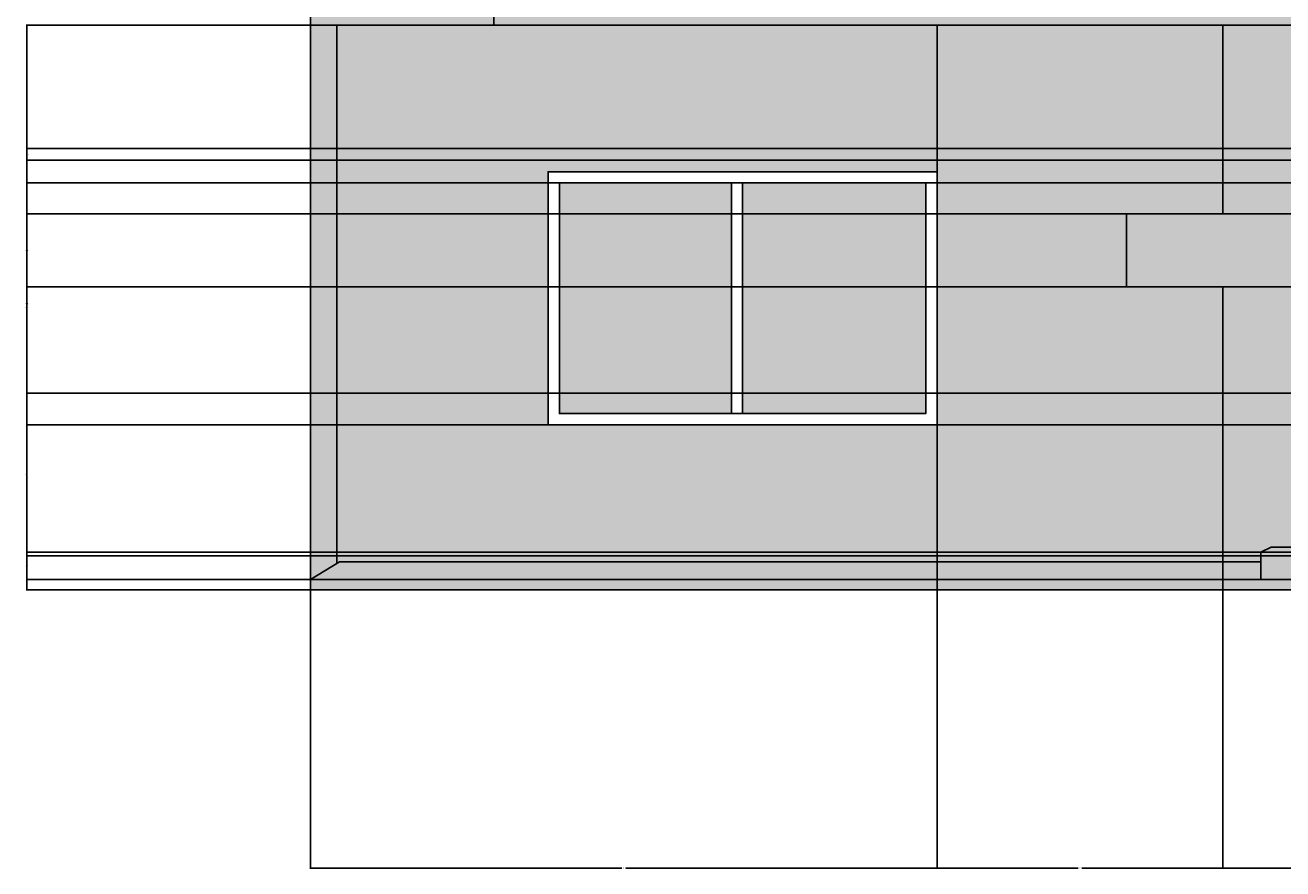
# Model space of a CAD drawing. Units: feet. Extents: x 2193 to 3502, y 890 to 1601.
# Tile 1 of 17: x 2193 to 2466, y 890 to 1073. Entities that reach past the tile are written whole.
import ezdxf

# ---------------------------------------------------------------- set-up
doc = ezdxf.new("R2010")
doc.units = ezdxf.units.FT
for name, color, linetype, lineweight in [('A-ANNO-DIMS', 2, 'Continuous', 18), ('A-ELEV', 7, 'Continuous', 25), ('A-ELEV-PATT', 8, 'Continuous', 13)]:
    doc.layers.add(name, color=color, linetype=linetype, lineweight=lineweight)
doc.styles.get("Standard").update_dxf_attribs({"font": 'arial.ttf'})
doc.dimstyles.get("Standard").update_dxf_attribs({"dimtxt": 0.18, "dimasz": 0.18, "dimexe": 0.18, "dimexo": 0.0625, "dimgap": 0.09, "dimtad": 0, "dimtih": 1, "dimtoh": 1, "dimdec": 0, "dimzin": 0, "dimdsep": 46, "dimlunit": 3, "dimtxsty": 'Standard', "dimcen": 0.09, "dimadec": 0, "dimazin": 0, "dimtfac": 1, "dimtdec": 0, "dimtofl": 0, "dimtmove": 0, "dimatfit": 3, "dimfxl": 1, "dimtolj": 1, "dimtzin": 0, "dimarcsym": 0})

# ---------------------------------------------------------------- blocks, each defined once
blk = doc.blocks.new('*D19')
at = {"layer": 'A-ANNO-DIMS', "color": 0, "lineweight": -2, "transparency": 16777216}
for p, q in [((2934.31, 1073.03), (2193.56, 1073.03)), ((2193.74, 1072.85), (2193.74, 1012.11)), ((2193.74, 951), (2193.74, 1011.75)), ((2934.31, 950.82), (2193.56, 950.82))]:
    blk.add_line(p, q, dxfattribs=at)
at = {"layer": 'A-ANNO-DIMS', "color": 0, "transparency": 16777216}
for points in [[(2193.71, 1072.85), (2193.77, 1072.85), (2193.74, 1073.03)], [(2193.71, 951), (2193.77, 951), (2193.74, 950.82)]]:
    blk.add_solid(points, dxfattribs=at)
at = {"layer": 'Defpoints', "color": 0, "transparency": 16777216}
for p in [(2193.74, 1073.03), (2934.37, 1073.03), (2934.37, 950.82)]:
    blk.add_point(p, dxfattribs=at)
at = {"layer": 'A-ANNO-DIMS', "color": 0, "transparency": 16777216, "insert": (2193.74, 1011.93), "char_height": 0.18, "attachment_point": 5}
blk.add_mtext('\\A1;122.2', dxfattribs=at)
blk = doc.blocks.new('*D23')
at = {"layer": 'A-ANNO-DIMS', "color": 0, "lineweight": -2, "transparency": 16777216}
for p, q in [((2988.24, 1038.87), (2193.56, 1038.87)), ((2193.74, 1038.69), (2193.74, 1012.87)), ((2193.74, 986.69), (2193.74, 1012.51)), ((2985.8, 986.51), (2193.56, 986.51))]:
    blk.add_line(p, q, dxfattribs=at)
at = {"layer": 'A-ANNO-DIMS', "color": 0, "transparency": 16777216}
for points in [[(2193.71, 1038.69), (2193.77, 1038.69), (2193.74, 1038.87)], [(2193.71, 986.69), (2193.77, 986.69), (2193.74, 986.51)]]:
    blk.add_solid(points, dxfattribs=at)
at = {"layer": 'Defpoints', "color": 0, "transparency": 16777216}
for p in [(2193.74, 1038.87), (2988.31, 1038.87), (2985.86, 986.51)]:
    blk.add_point(p, dxfattribs=at)
at = {"layer": 'A-ANNO-DIMS', "color": 0, "transparency": 16777216, "insert": (2193.74, 1012.69), "char_height": 0.18, "attachment_point": 5}
blk.add_mtext('\\A1;52.35', dxfattribs=at)
blk = doc.blocks.new('*D26')
at = {"layer": 'A-ANNO-DIMS', "color": 0, "lineweight": -2, "transparency": 16777216}
for p, q in [((2255.16, 950.89), (2255.16, 1601.47)), ((2255.34, 1601.29), (2507.42, 1601.29)), ((2760.29, 1601.29), (2508.21, 1601.29)), ((2760.47, 1541.11), (2760.47, 1601.47))]:
    blk.add_line(p, q, dxfattribs=at)
at = {"layer": 'A-ANNO-DIMS', "color": 0, "transparency": 16777216}
for points in [[(2255.34, 1601.32), (2255.34, 1601.26), (2255.16, 1601.29)], [(2760.29, 1601.32), (2760.29, 1601.26), (2760.47, 1601.29)]]:
    blk.add_solid(points, dxfattribs=at)
at = {"layer": 'Defpoints', "color": 0, "transparency": 16777216}
for p in [(2760.47, 1601.29), (2760.47, 1541.04), (2255.16, 950.82)]:
    blk.add_point(p, dxfattribs=at)
at = {"layer": 'A-ANNO-DIMS', "color": 0, "transparency": 16777216, "insert": (2507.82, 1601.29), "char_height": 0.18, "attachment_point": 5}
blk.add_mtext('\\A1;505.3', dxfattribs=at)
blk = doc.blocks.new('*D27')
at = {"layer": 'A-ANNO-DIMS', "color": 0, "lineweight": -2, "transparency": 16777216}
for p, q in [((2390.89, 956.87), (2390.89, 890.39)), ((2255.16, 950.76), (2255.16, 890.39)), ((2255.34, 890.57), (2322.57, 890.57)), ((2390.71, 890.57), (2323.48, 890.57))]:
    blk.add_line(p, q, dxfattribs=at)
at = {"layer": 'A-ANNO-DIMS', "color": 0, "transparency": 16777216}
for points in [[(2255.34, 890.6), (2255.34, 890.54), (2255.16, 890.57)], [(2390.71, 890.6), (2390.71, 890.54), (2390.89, 890.57)]]:
    blk.add_solid(points, dxfattribs=at)
at = {"layer": 'Defpoints', "color": 0, "transparency": 16777216}
for p in [(2390.89, 956.94), (2255.16, 950.82), (2390.89, 890.57)]:
    blk.add_point(p, dxfattribs=at)
at = {"layer": 'A-ANNO-DIMS', "color": 0, "transparency": 16777216, "insert": (2323.03, 890.57), "char_height": 0.18, "attachment_point": 5}
blk.add_mtext('\\A1;135.74', dxfattribs=at)
blk = doc.blocks.new('*D28')
at = {"layer": 'A-ANNO-DIMS', "color": 0, "lineweight": -2, "transparency": 16777216}
for p, q in [((2390.89, 956.87), (2390.89, 890.39)), ((2452.78, 956.87), (2452.78, 890.39)), ((2391.07, 890.57), (2421.44, 890.57)), ((2452.6, 890.57), (2422.23, 890.57))]:
    blk.add_line(p, q, dxfattribs=at)
at = {"layer": 'A-ANNO-DIMS', "color": 0, "transparency": 16777216}
for points in [[(2391.07, 890.6), (2391.07, 890.54), (2390.89, 890.57)], [(2452.6, 890.6), (2452.6, 890.54), (2452.78, 890.57)]]:
    blk.add_solid(points, dxfattribs=at)
at = {"layer": 'Defpoints', "color": 0, "transparency": 16777216}
for p in [(2390.89, 956.94), (2452.78, 956.94), (2452.78, 890.57)]:
    blk.add_point(p, dxfattribs=at)
at = {"layer": 'A-ANNO-DIMS', "color": 0, "transparency": 16777216, "insert": (2421.84, 890.57), "char_height": 0.18, "attachment_point": 5}
blk.add_mtext('\\A1;61.89', dxfattribs=at)
blk = doc.blocks.new('*D29')
at = {"layer": 'A-ANNO-DIMS', "color": 0, "lineweight": -2, "transparency": 16777216}
for p, q in [((2452.78, 956.87), (2452.78, 890.39)), ((2626.2, 950.76), (2626.2, 890.39)), ((2452.96, 890.57), (2539.1, 890.57)), ((2626.02, 890.57), (2539.87, 890.57))]:
    blk.add_line(p, q, dxfattribs=at)
at = {"layer": 'A-ANNO-DIMS', "color": 0, "transparency": 16777216}
for points in [[(2452.96, 890.6), (2452.96, 890.54), (2452.78, 890.57)], [(2626.02, 890.6), (2626.02, 890.54), (2626.2, 890.57)]]:
    blk.add_solid(points, dxfattribs=at)
at = {"layer": 'Defpoints', "color": 0, "transparency": 16777216}
for p in [(2452.78, 956.94), (2626.2, 950.82), (2626.2, 890.57)]:
    blk.add_point(p, dxfattribs=at)
at = {"layer": 'A-ANNO-DIMS', "color": 0, "transparency": 16777216, "insert": (2539.49, 890.57), "char_height": 0.18, "attachment_point": 5}
blk.add_mtext('\\A1;173.4', dxfattribs=at)
blk = doc.blocks.new('*D32')
at = {"layer": 'A-ANNO-DIMS', "color": 0, "lineweight": -2, "transparency": 16777216}
for p, q in [((2255.09, 1073.03), (2193.56, 1073.03)), ((2193.74, 1072.85), (2193.74, 1012.11)), ((2193.74, 951), (2193.74, 1011.75)), ((2255.09, 950.82), (2193.56, 950.82))]:
    blk.add_line(p, q, dxfattribs=at)
at = {"layer": 'A-ANNO-DIMS', "color": 0, "transparency": 16777216}
for points in [[(2193.71, 1072.85), (2193.77, 1072.85), (2193.74, 1073.03)], [(2193.71, 951), (2193.77, 951), (2193.74, 950.82)]]:
    blk.add_solid(points, dxfattribs=at)
at = {"layer": 'Defpoints', "color": 0, "transparency": 16777216}
for p in [(2193.74, 1073.03), (2255.16, 1073.03), (2255.16, 950.82)]:
    blk.add_point(p, dxfattribs=at)
at = {"layer": 'A-ANNO-DIMS', "color": 0, "transparency": 16777216, "insert": (2193.74, 1011.93), "char_height": 0.18, "attachment_point": 5}
blk.add_mtext('\\A1;122.2', dxfattribs=at)
blk = doc.blocks.new('*D98')
at = {"layer": 'A-ANNO-DIMS', "color": 0, "lineweight": -2, "transparency": 16777216}
for p, q in [((3111.07, 1032.19), (2193.56, 1032.19)), ((2193.74, 1032.01), (2193.74, 1024.48)), ((2193.74, 1016.58), (2193.74, 1024.11)), ((3111.07, 1016.4), (2193.56, 1016.4))]:
    blk.add_line(p, q, dxfattribs=at)
at = {"layer": 'A-ANNO-DIMS', "color": 0, "transparency": 16777216}
for points in [[(2193.71, 1032.01), (2193.77, 1032.01), (2193.74, 1032.19)], [(2193.71, 1016.58), (2193.77, 1016.58), (2193.74, 1016.4)]]:
    blk.add_solid(points, dxfattribs=at)
at = {"layer": 'Defpoints', "color": 0, "transparency": 16777216}
for p in [(2193.74, 1032.19), (3111.13, 1032.19), (3111.13, 1016.4)]:
    blk.add_point(p, dxfattribs=at)
at = {"layer": 'A-ANNO-DIMS', "color": 0, "transparency": 16777216, "insert": (2193.74, 1024.3), "char_height": 0.18, "attachment_point": 5}
blk.add_mtext('\\A1;15.793', dxfattribs=at)
blk = doc.blocks.new('*D116')
at = {"layer": 'A-ANNO-DIMS', "color": 0, "lineweight": -2, "transparency": 16777216}
for p, q in [((3140.16, 958.96), (2193.56, 958.96)), ((2193.74, 958.78), (2193.74, 956.18)), ((2193.74, 953.21), (2193.74, 955.81)), ((3140.16, 953.03), (2193.56, 953.03))]:
    blk.add_line(p, q, dxfattribs=at)
at = {"layer": 'A-ANNO-DIMS', "color": 0, "transparency": 16777216}
for points in [[(2193.71, 958.78), (2193.77, 958.78), (2193.74, 958.96)], [(2193.71, 953.21), (2193.77, 953.21), (2193.74, 953.03)]]:
    blk.add_solid(points, dxfattribs=at)
at = {"layer": 'Defpoints', "color": 0, "transparency": 16777216}
for p in [(2193.74, 958.96), (3140.22, 958.96), (3140.22, 953.03)]:
    blk.add_point(p, dxfattribs=at)
at = {"layer": 'A-ANNO-DIMS', "color": 0, "transparency": 16777216, "insert": (2193.74, 955.99), "char_height": 0.18, "attachment_point": 5}
blk.add_mtext('\\A1;5.924', dxfattribs=at)
blk = doc.blocks.new('*D124')
at = {"layer": 'A-ANNO-DIMS', "color": 0, "lineweight": -2, "transparency": 16777216}
for p, q in [((3304.91, 1046.36), (2193.56, 1046.36)), ((2193.74, 1046.18), (2193.74, 1045.26)), ((3304.91, 1043.78), (2193.56, 1043.78)), ((2193.74, 1043.96), (2193.74, 1044.89))]:
    blk.add_line(p, q, dxfattribs=at)
at = {"layer": 'A-ANNO-DIMS', "color": 0, "transparency": 16777216}
for points in [[(2193.71, 1046.18), (2193.77, 1046.18), (2193.74, 1046.36)], [(2193.71, 1043.96), (2193.77, 1043.96), (2193.74, 1043.78)]]:
    blk.add_solid(points, dxfattribs=at)
at = {"layer": 'Defpoints', "color": 0, "transparency": 16777216}
for p in [(3304.97, 1046.36), (2193.74, 1043.78), (3304.97, 1043.78)]:
    blk.add_point(p, dxfattribs=at)
at = {"layer": 'A-ANNO-DIMS', "color": 0, "transparency": 16777216, "insert": (2193.74, 1045.07), "char_height": 0.18, "attachment_point": 5}
blk.add_mtext('\\A1;2.583', dxfattribs=at)
blk = doc.blocks.new('*D130')
at = {"layer": 'A-ANNO-DIMS', "color": 0, "lineweight": -2, "transparency": 16777216}
for p, q in [((3304.91, 993.39), (2193.56, 993.39)), ((2193.74, 993.21), (2193.74, 975.95)), ((2193.74, 958.33), (2193.74, 975.59)), ((3304.91, 958.15), (2193.56, 958.15))]:
    blk.add_line(p, q, dxfattribs=at)
at = {"layer": 'A-ANNO-DIMS', "color": 0, "transparency": 16777216}
for points in [[(2193.71, 993.21), (2193.77, 993.21), (2193.74, 993.39)], [(2193.71, 958.33), (2193.77, 958.33), (2193.74, 958.15)]]:
    blk.add_solid(points, dxfattribs=at)
at = {"layer": 'Defpoints', "color": 0, "transparency": 16777216}
for p in [(2193.74, 993.39), (3304.97, 993.39), (3304.97, 958.15)]:
    blk.add_point(p, dxfattribs=at)
at = {"layer": 'A-ANNO-DIMS', "color": 0, "transparency": 16777216, "insert": (2193.74, 975.77), "char_height": 0.18, "attachment_point": 5}
blk.add_mtext('\\A1;35.24', dxfattribs=at)

msp = doc.modelspace()

# ---------------------------------------------------------------- hatches: boundary and pattern name
at = {"layer": 'A-ELEV-PATT'}
h = msp.add_hatch(color=256, dxfattribs=at)
h.dxf.hatch_style = 1
h.paths.add_polyline_path([(2390.8933, 1367.5739), (2294.8992, 1367.5739), (2294.8992, 1329.5765), (2390.8933, 1329.5765)])
h.paths.add_polyline_path([(2489.6169, 1055.3069), (2585.8844, 1055.3069), (2585.8844, 1032.1935), (2620.0491, 1032.1935), (2620.0491, 1073.031), (2452.7821, 1073.031), (2452.7821, 1032.1935), (2489.6169, 1032.1935)])
h.paths.add_polyline_path([(2754.7661, 1073.031), (2654.2841, 1073.031), (2654.2841, 1047.0961), (2754.7661, 1047.0961)])
h.paths.add_polyline_path([(2643.9681, 1484.1152), (2699.5726, 1484.1152), (2699.5726, 1502.0763), (2602.8648, 1502.0763), (2602.8648, 1408.4814), (2643.9681, 1408.4814)])
h.paths.add_polyline_path([(2699.6322, 1367.5739), (2646.2844, 1367.5739), (2646.2844, 1268.6599), (2647.1841, 1268.6599), (2647.1841, 1329.5765), (2699.6322, 1329.5765)])
h.paths.add_polyline_path([(2699.6322, 1224.865), (2616.5596, 1224.865), (2616.5596, 1133.8558), (2647.1841, 1133.8558), (2647.1841, 1194.7724), (2699.6322, 1194.7724)])
h = msp.add_hatch(color=256, dxfattribs=at)
h.dxf.hatch_style = 1
h.paths.add_polyline_path([(2760.4733, 956.8829), (2754.7661, 956.8829), (2625.7563, 956.8829), (2626.1971, 953.031), (2626.1971, 950.8228), (2762.2048, 950.8228)])
h.paths.add_polyline_path([(2587.7084, 958.9555), (2461.0056, 958.9555), (2461.0056, 953.031), (2587.7084, 953.031)])
h.paths.add_polyline_path([(2480.0809, 960.0129), (2463.2716, 960.0129), (2461.0056, 958.9555), (2480.0809, 958.9555)])
h.paths.add_polyline_path([(2514.917, 960.0129), (2500.4779, 960.0129), (2500.4779, 958.9555), (2514.917, 958.9555)])
h.paths.add_polyline_path([(2552.6959, 960.0129), (2538.2568, 960.0129), (2538.2568, 958.9555), (2552.6959, 958.9555)])
h.paths.add_polyline_path([(2588.4279, 960.0129), (2573.0929, 960.0129), (2573.0929, 958.9555), (2587.7084, 958.9555)])
h.paths.add_polyline_path([(2588.4279, 960.0129), (2587.7084, 958.9555), (2587.7084, 953.031), (2588.4279, 953.031)])
h.paths.add_polyline_path([(2461.0056, 956.8829), (2261.443, 956.8829), (2255.1574, 953.031), (2461.0056, 953.031)])
h.paths.add_polyline_path([(2625.7563, 956.8829), (2600.3918, 956.8829), (2600.3918, 953.031), (2626.1971, 953.031)])
h.paths.add_polyline_path([(2600.3918, 956.8829), (2588.4279, 956.8829), (2588.4279, 953.031), (2600.3918, 953.031)])
h.paths.add_polyline_path([(2602.8648, 1494.8043), (2286.5029, 1494.8043), (2286.5029, 1492.5146), (2602.8648, 1492.5146)])
h.paths.add_polyline_path([(2322.8578, 1492.5146), (2319.4392, 1492.5146), (2337.7496, 1475.8561), (2341.1681, 1475.8561)])
h.paths.add_polyline_path([(2341.1681, 1475.8561), (2337.7496, 1475.8561), (2341.051, 1472.8525), (2344.4696, 1472.8525)])
h.paths.add_polyline_path([(2344.4696, 1472.8525), (2341.051, 1472.8525), (2352.3124, 1462.6071), (2355.731, 1462.6071)])
h.paths.add_polyline_path([(2355.731, 1462.6071), (2352.3124, 1462.6071), (2355.6139, 1459.6035), (2359.0325, 1459.6035)])
h.paths.add_polyline_path([(2325.1721, 1459.1592), (2323.1659, 1459.1592), (2323.1659, 1408.4814), (2325.1721, 1408.4814)])
h.paths.add_polyline_path([(2297.6937, 1482.3334), (2295.7368, 1484.1138), (2295.7368, 1408.4814), (2297.6937, 1408.4814)])
h.paths.add_polyline_path([(2300.8766, 1479.4377), (2297.6937, 1482.3334), (2297.6937, 1408.4814), (2300.8766, 1408.4814)])
h.paths.add_polyline_path([(2337.7496, 1475.8561), (2304.8133, 1475.8561), (2308.1148, 1472.8525), (2341.051, 1472.8525)])
h.paths.add_polyline_path([(2352.3124, 1462.6071), (2319.3762, 1462.6071), (2322.6776, 1459.6035), (2355.6139, 1459.6035)])
h.paths.add_polyline_path([(2374.1044, 1475.8561), (2341.1681, 1475.8561), (2344.4696, 1472.8525), (2377.4059, 1472.8525)])
h.paths.add_polyline_path([(2388.6672, 1462.6071), (2355.731, 1462.6071), (2359.0325, 1459.6035), (2391.9687, 1459.6035)])
h.paths.add_polyline_path([(2392.0858, 1462.6071), (2388.6672, 1462.6071), (2391.9687, 1459.6035), (2395.3873, 1459.6035)])
h.paths.add_polyline_path([(2380.8245, 1472.8525), (2377.4059, 1472.8525), (2388.6672, 1462.6071), (2392.0858, 1462.6071)])
h.paths.add_polyline_path([(2377.523, 1475.8561), (2374.1044, 1475.8561), (2377.4059, 1472.8525), (2380.8245, 1472.8525)])
h.paths.add_polyline_path([(2359.2126, 1492.5146), (2355.794, 1492.5146), (2374.1044, 1475.8561), (2377.523, 1475.8561)])
h.paths.add_polyline_path([(2395.5674, 1492.5146), (2392.1488, 1492.5146), (2410.4592, 1475.8561), (2413.8778, 1475.8561)])
h.paths.add_polyline_path([(2410.4592, 1475.8561), (2377.523, 1475.8561), (2380.8245, 1472.8525), (2413.7607, 1472.8525)])
h.paths.add_polyline_path([(2413.8778, 1475.8561), (2410.4592, 1475.8561), (2413.7607, 1472.8525), (2417.1793, 1472.8525)])
h.paths.add_polyline_path([(2417.1793, 1472.8525), (2413.7607, 1472.8525), (2425.022, 1462.6071), (2428.4406, 1462.6071)])
h.paths.add_polyline_path([(2425.022, 1462.6071), (2392.0858, 1462.6071), (2395.3873, 1459.6035), (2428.3235, 1459.6035)])
h.paths.add_polyline_path([(2428.4406, 1462.6071), (2425.022, 1462.6071), (2428.3235, 1459.6035), (2431.7421, 1459.6035)])
h.paths.add_polyline_path([(2461.3769, 1462.6071), (2428.4406, 1462.6071), (2431.7421, 1459.6035), (2464.6784, 1459.6035)])
h.paths.add_polyline_path([(2577.3415, 1492.5146), (2573.9229, 1492.5146), (2591.9256, 1476.1361), (2593.2177, 1478.0707)])
h.paths.add_polyline_path([(2540.9867, 1492.5146), (2537.5681, 1492.5146), (2555.8785, 1475.8561), (2559.2971, 1475.8561)])
h.paths.add_polyline_path([(2591.7386, 1475.8561), (2559.2971, 1475.8561), (2562.5986, 1472.8525), (2589.7325, 1472.8525)])
h.paths.add_polyline_path([(2555.8785, 1475.8561), (2522.9423, 1475.8561), (2526.2437, 1472.8525), (2559.18, 1472.8525)])
h.paths.add_polyline_path([(2559.2971, 1475.8561), (2555.8785, 1475.8561), (2559.18, 1472.8525), (2562.5986, 1472.8525)])
h.paths.add_polyline_path([(2562.5986, 1472.8525), (2559.18, 1472.8525), (2570.4413, 1462.6071), (2573.8599, 1462.6071)])
h.paths.add_polyline_path([(2570.4413, 1462.6071), (2537.5051, 1462.6071), (2540.8066, 1459.6035), (2573.7428, 1459.6035)])
h.paths.add_polyline_path([(2582.8896, 1462.6071), (2573.8599, 1462.6071), (2577.1614, 1459.6035), (2580.8835, 1459.6035)])
h.paths.add_polyline_path([(2573.8599, 1462.6071), (2570.4413, 1462.6071), (2573.7428, 1459.6035), (2577.1614, 1459.6035)])
h.paths.add_polyline_path([(2591.7386, 1475.8561), (2589.7325, 1472.8525), (2589.7325, 1408.4814), (2591.7386, 1408.4814)])
h.paths.add_polyline_path([(2582.8896, 1462.6071), (2580.8835, 1459.6035), (2580.8835, 1408.4814), (2582.8896, 1408.4814)])
h.paths.add_polyline_path([(2504.6319, 1492.5146), (2501.2133, 1492.5146), (2519.5237, 1475.8561), (2522.9423, 1475.8561)])
h.paths.add_polyline_path([(2534.0865, 1462.6071), (2501.1503, 1462.6071), (2504.4518, 1459.6035), (2537.388, 1459.6035)])
h.paths.add_polyline_path([(2537.5051, 1462.6071), (2534.0865, 1462.6071), (2537.388, 1459.6035), (2540.8066, 1459.6035)])
h.paths.add_polyline_path([(2526.2437, 1472.8525), (2522.8252, 1472.8525), (2534.0865, 1462.6071), (2537.5051, 1462.6071)])
h.paths.add_polyline_path([(2522.9423, 1475.8561), (2519.5237, 1475.8561), (2522.8252, 1472.8525), (2526.2437, 1472.8525)])
h.paths.add_polyline_path([(2519.5237, 1475.8561), (2486.5874, 1475.8561), (2489.8889, 1472.8525), (2522.8252, 1472.8525)])
h.paths.add_polyline_path([(2483.1689, 1475.8561), (2450.2326, 1475.8561), (2453.5341, 1472.8525), (2486.4703, 1472.8525)])
h.paths.add_polyline_path([(2486.5874, 1475.8561), (2483.1689, 1475.8561), (2486.4703, 1472.8525), (2489.8889, 1472.8525)])
h.paths.add_polyline_path([(2468.277, 1492.5146), (2464.8585, 1492.5146), (2483.1689, 1475.8561), (2486.5874, 1475.8561)])
h.paths.add_polyline_path([(2489.8889, 1472.8525), (2486.4703, 1472.8525), (2497.7317, 1462.6071), (2501.1503, 1462.6071)])
h.paths.add_polyline_path([(2497.7317, 1462.6071), (2464.7955, 1462.6071), (2468.0969, 1459.6035), (2501.0332, 1459.6035)])
h.paths.add_polyline_path([(2501.1503, 1462.6071), (2497.7317, 1462.6071), (2501.0332, 1459.6035), (2504.4518, 1459.6035)])
h.paths.add_polyline_path([(2464.7955, 1462.6071), (2461.3769, 1462.6071), (2464.6784, 1459.6035), (2468.0969, 1459.6035)])
h.paths.add_polyline_path([(2453.5341, 1472.8525), (2450.1155, 1472.8525), (2461.3769, 1462.6071), (2464.7955, 1462.6071)])
h.paths.add_polyline_path([(2431.9222, 1492.5146), (2428.5036, 1492.5146), (2446.814, 1475.8561), (2450.2326, 1475.8561)])
h.paths.add_polyline_path([(2446.814, 1475.8561), (2413.8778, 1475.8561), (2417.1793, 1472.8525), (2450.1155, 1472.8525)])
h.paths.add_polyline_path([(2450.2326, 1475.8561), (2446.814, 1475.8561), (2450.1155, 1472.8525), (2453.5341, 1472.8525)])
h.paths.add_polyline_path([(2407.5925, 1459.1592), (2405.5863, 1459.1592), (2405.5863, 1408.4814), (2407.5925, 1408.4814)])
h.paths.add_polyline_path([(2499.2252, 1459.1592), (2497.2191, 1459.1592), (2497.2191, 1408.4814), (2499.2252, 1408.4814)])
h = msp.add_hatch(color=256, dxfattribs=at)
h.dxf.hatch_style = 1
h.paths.add_polyline_path([(2294.8992, 1367.5739), (2275.0482, 1367.5739), (2275.0482, 1382.0763), (2536.5416, 1382.0763), (2536.5416, 1406.15), (2256.3232, 1406.15), (2256.3232, 1089.3627), (2255.1574, 1089.3627), (2255.1574, 1073.031), (2294.8992, 1073.031)])
h.paths.add_polyline_path([(2517.7591, 1241.1967), (2468.2854, 1241.1967), (2468.2854, 1224.865), (2598.591, 1224.865), (2598.591, 1233.561), (2517.7591, 1233.561)])
h.paths.add_polyline_path([(2699.6322, 1241.1967), (2636.5184, 1241.1967), (2636.5184, 1233.561), (2616.5596, 1233.561), (2616.5596, 1224.865), (2699.6322, 1224.865)])
h.paths.add_polyline_path([(2615.4622, 1233.561), (2613.8564, 1233.561), (2613.8564, 1224.865), (2615.4622, 1224.865)])
h.paths.add_polyline_path([(2612.759, 1233.561), (2609.5836, 1233.561), (2609.5836, 1224.865), (2612.759, 1224.865)])
h.paths.add_polyline_path([(2608.4862, 1233.561), (2606.5316, 1233.561), (2606.5316, 1224.865), (2608.4862, 1224.865)])
h.paths.add_polyline_path([(2605.4342, 1233.561), (2602.5204, 1233.561), (2602.5204, 1224.865), (2605.4342, 1224.865)])
h.paths.add_polyline_path([(2601.423, 1233.561), (2599.6883, 1233.561), (2599.6883, 1224.865), (2601.423, 1224.865)])
h.paths.add_polyline_path([(2517.7591, 1089.3627), (2468.2854, 1089.3627), (2468.2854, 1079.031), (2294.8992, 1079.031), (2294.8992, 1073.031), (2390.8933, 1073.031), (2452.7821, 1073.031), (2760.4733, 1073.031), (2760.4733, 1089.3627), (2699.6322, 1089.3627), (2636.5184, 1089.3627), (2636.5184, 1081.7269), (2517.7591, 1081.7269)])
h = msp.add_hatch(color=256, dxfattribs=at)
h.dxf.hatch_style = 1
h.paths.add_polyline_path([(2576.3428, 1407.7384), (2536.5416, 1407.7384), (2536.5416, 1406.15), (2536.5416, 1382.0763), (2576.3428, 1382.0763)])
h.paths.add_polyline_path([(2627.3548, 1407.7384), (2576.5924, 1407.7384), (2576.5924, 1382.0763), (2627.3548, 1382.0763)])
h.paths.add_polyline_path([(2667.9236, 1407.7384), (2627.6045, 1407.7384), (2627.6045, 1382.0763), (2667.9236, 1382.0763)])
h.paths.add_polyline_path([(2699.6322, 1407.7384), (2668.1733, 1407.7384), (2668.1733, 1382.0763), (2699.6322, 1382.0763)])
h.paths.add_polyline_path([(2497.5717, 1323.2248), (2470.7305, 1323.2248), (2470.7305, 1271.105), (2497.5717, 1271.105)])
h.paths.add_polyline_path([(2577.3219, 1323.2248), (2500.599, 1323.2248), (2500.599, 1271.105), (2577.3219, 1271.105)])
h.paths.add_polyline_path([(2388.4482, 1327.1314), (2343.4244, 1327.1314), (2343.4244, 1268.6599), (2388.4482, 1268.6599)])
h.paths.add_polyline_path([(2342.3682, 1327.1314), (2297.3443, 1327.1314), (2297.3443, 1268.6599), (2342.3682, 1268.6599)])
h.paths.add_polyline_path([(2335.8632, 1214.8367), (2301.4984, 1214.8367), (2301.4984, 1133.1367), (2335.8632, 1133.1367)])
h.paths.add_polyline_path([(2371.1246, 1214.8367), (2337.2323, 1214.8367), (2337.2323, 1133.1367), (2371.1246, 1133.1367)])
h.paths.add_polyline_path([(2390.8933, 1214.8367), (2372.4936, 1214.8367), (2372.4936, 1133.1367), (2390.8933, 1133.1367)])
h.paths.add_polyline_path([(2577.3219, 1188.4208), (2500.599, 1188.4208), (2500.599, 1136.3009), (2577.3219, 1136.3009)])
h.paths.add_polyline_path([(2497.5717, 1188.4208), (2470.7305, 1188.4208), (2470.7305, 1136.3009), (2497.5717, 1136.3009)])
h.paths.add_polyline_path([(2381.4675, 1132.3937), (2301.4984, 1132.3937), (2301.4984, 1085.6301), (2381.4675, 1085.6301)])
h.paths.add_polyline_path([(2461.6863, 1132.3937), (2381.7172, 1132.3937), (2381.7172, 1085.6301), (2461.6863, 1085.6301)])
h.paths.add_polyline_path([(2494.0463, 1133.1128), (2468.2854, 1133.1128), (2468.2854, 1089.3627), (2494.0463, 1089.3627)])
h.paths.add_polyline_path([(2517.7591, 1133.1128), (2494.296, 1133.1128), (2494.296, 1089.3627), (2517.7591, 1089.3627)])
h.paths.add_polyline_path([(2667.9236, 1133.1128), (2636.5184, 1133.1128), (2636.5184, 1089.3627), (2667.9236, 1089.3627)])
h.paths.add_polyline_path([(2699.6322, 1133.1128), (2668.1733, 1133.1128), (2668.1733, 1089.3627), (2699.6322, 1089.3627)])
h.paths.add_polyline_path([(2651.839, 1070.5859), (2638.7977, 1070.5859), (2638.7977, 1047.0961), (2651.839, 1047.0961)])
h.paths.add_polyline_path([(2637.6317, 1070.5859), (2625.7563, 1070.5859), (2625.7563, 1047.0961), (2637.6317, 1047.0961)])
h.paths.add_polyline_path([(2583.4393, 1052.8618), (2515.9216, 1052.8618), (2515.9216, 1032.1935), (2583.4393, 1032.1935)])
h.paths.add_polyline_path([(2514.4293, 1052.8618), (2492.062, 1052.8618), (2492.062, 1032.1935), (2514.4293, 1032.1935)])
h.paths.add_polyline_path([(2388.4482, 1038.8658), (2348.7682, 1038.8658), (2348.7682, 988.9597), (2388.4482, 988.9597)])
h.paths.add_polyline_path([(2346.3231, 1038.8658), (2309.0883, 1038.8658), (2309.0883, 988.9597), (2346.3231, 988.9597)])
h.paths.add_polyline_path([(2667.9236, 1267.9169), (2636.5184, 1267.9169), (2636.5184, 1241.1967), (2667.9236, 1241.1967)])
h.paths.add_polyline_path([(2699.6322, 1267.9169), (2668.1733, 1267.9169), (2668.1733, 1241.1967), (2699.6322, 1241.1967)])
h.paths.add_polyline_path([(2517.7591, 1267.9169), (2494.296, 1267.9169), (2494.296, 1241.1967), (2517.7591, 1241.1967)])
h.paths.add_polyline_path([(2494.0463, 1267.9169), (2468.2854, 1267.9169), (2468.2854, 1266.7092), (2468.2854, 1241.1967), (2494.0463, 1241.1967)])
h = msp.add_hatch(color=256, dxfattribs=at)
h.dxf.hatch_style = 1
h.paths.add_polyline_path([(2452.7821, 1355.2199), (2622.9814, 1355.2199), (2622.9814, 1268.6599), (2646.2844, 1268.6599), (2646.2844, 1367.5739), (2390.8933, 1367.5739), (2390.8933, 1268.6599), (2452.7821, 1268.6599)])
h.paths.add_polyline_path([(2452.7821, 1016.4), (2431.9134, 1016.4), (2431.9134, 1032.1935), (2452.7821, 1032.1935), (2452.7821, 1073.031), (2390.8933, 1073.031), (2390.8933, 956.8829), (2452.7821, 956.8829)])
h.paths.add_polyline_path([(2452.7821, 1241.1967), (2390.8933, 1241.1967), (2390.8933, 1133.1367), (2452.7821, 1133.1367)])
h.paths.add_polyline_path([(2636.5184, 1267.9169), (2517.7591, 1267.9169), (2517.7591, 1233.561), (2598.591, 1233.561), (2598.591, 1249.8256), (2599.6883, 1249.8256), (2599.6883, 1233.561), (2601.423, 1233.561), (2601.423, 1247.0422), (2602.5204, 1247.0422), (2602.5204, 1233.561), (2605.4342, 1233.561), (2605.4342, 1250.4403), (2606.5316, 1250.4403), (2606.5316, 1233.561), (2608.4862, 1233.561), (2608.4862, 1248.4363), (2609.5836, 1248.4363), (2609.5836, 1233.561), (2612.759, 1233.561), (2612.759, 1243.2956), (2613.8564, 1243.2956), (2613.8564, 1233.561), (2615.4622, 1233.561), (2615.4622, 1249.6561), (2616.5596, 1249.6561), (2616.5596, 1233.561), (2636.5184, 1233.561)])
h.paths.add_polyline_path([(2601.423, 1133.1128), (2599.6883, 1133.1128), (2599.6883, 1115.2331), (2598.591, 1115.2331), (2598.591, 1133.1128), (2517.7591, 1133.1128), (2517.7591, 1081.7269), (2636.5184, 1081.7269), (2636.5184, 1133.1128), (2616.5596, 1133.1128), (2616.5596, 1115.0637), (2615.4622, 1115.0637), (2615.4622, 1133.1128), (2613.8564, 1133.1128), (2613.8564, 1108.7032), (2612.759, 1108.7032), (2612.759, 1133.1128), (2609.5836, 1133.1128), (2609.5836, 1113.8439), (2608.4862, 1113.8439), (2608.4862, 1133.1128), (2606.5316, 1133.1128), (2606.5316, 1115.8479), (2605.4342, 1115.8479), (2605.4342, 1133.1128), (2602.5204, 1133.1128), (2602.5204, 1112.4498), (2601.423, 1112.4498)])
h = msp.add_hatch(color=256, dxfattribs=at)
h.dxf.hatch_style = 1
h.paths.add_polyline_path([(2760.4733, 1073.031), (2754.7661, 1073.031), (2754.7661, 956.8829), (2760.4733, 956.8829)])
h.paths.add_polyline_path([(2625.7563, 1073.031), (2620.0491, 1073.031), (2620.0491, 1032.1935), (2625.7563, 1032.1935), (2625.7563, 1047.0961)])
h.paths.add_polyline_path([(2260.8647, 1073.031), (2255.1574, 1073.031), (2255.1574, 953.031), (2260.8647, 956.5285)])
h = msp.add_hatch(color=256, dxfattribs=at)
h.dxf.hatch_style = 1
h.paths.add_polyline_path([(2390.8933, 1073.031), (2260.8647, 1073.031), (2260.8647, 956.5285), (2261.443, 956.8829), (2390.8933, 956.8829), (2390.8933, 986.5146), (2306.6431, 986.5146), (2306.6431, 1041.3109), (2390.8933, 1041.3109)])
h = msp.add_hatch(color=256, dxfattribs=at)
h.dxf.hatch_style = 1
h.paths.add_polyline_path([(2625.7563, 1032.1935), (2431.9134, 1032.1935), (2431.9134, 1016.4), (2600.3918, 1016.4), (2600.3918, 956.8829), (2625.7563, 956.8829)])
h = msp.add_hatch(color=256, dxfattribs=at)
h.dxf.hatch_style = 1
h.paths.add_polyline_path([(2514.917, 1014.5106), (2513.3297, 1014.5106), (2513.3297, 1016.4), (2452.7821, 1016.4), (2452.7821, 956.8829), (2461.0056, 956.8829), (2461.0056, 958.9555), (2463.2716, 960.0129), (2480.0809, 960.0129), (2480.0809, 999.2439), (2478.6095, 999.2439), (2478.6095, 1001.1334), (2501.9493, 1001.1334), (2501.9493, 999.2439), (2500.4779, 999.2439), (2500.4779, 960.0129), (2514.917, 960.0129)])
h.paths.add_polyline_path([(2552.6959, 999.2439), (2551.2245, 999.2439), (2551.2245, 1001.1334), (2574.5643, 1001.1334), (2574.5643, 999.2439), (2573.0929, 999.2439), (2573.0929, 958.9555), (2587.7084, 958.9555), (2587.7084, 953.031), (2600.3918, 953.031), (2600.3918, 1016.4), (2539.8441, 1016.4), (2539.8441, 1014.5106), (2538.2568, 1014.5106), (2538.2568, 960.0129), (2552.6959, 960.0129)])
h = msp.add_hatch(color=256, dxfattribs=at)
h.dxf.hatch_style = 1
h.paths.add_polyline_path([(2626.1971, 953.031), (2255.1574, 953.031), (2255.1574, 950.8228), (2626.1971, 950.8228)])

# ---------------------------------------------------------------- linework, layer by layer
at = {"layer": 'A-ELEV'}
for p, q in [((2255.1574, 953.031), (2255.1574, 1089.3627)), ((2255.1574, 1073.031), (2760.4733, 1073.031)), ((2461.0056, 958.9555), (2463.2716, 960.0129)), ((2463.2716, 960.0129), (2480.0809, 960.0129)), ((2255.1574, 953.031), (2261.443, 956.8829)), ((2261.443, 956.8829), (2461.0056, 956.8829)), ((2255.1574, 953.031), (2626.1971, 953.031)), ((2255.1574, 953.031), (2255.1574, 950.8228)), ((2255.1574, 950.8228), (2626.1971, 950.8228))]:
    msp.add_line(p, q, dxfattribs=at)
for points in [[(2760.4733, 1494.0584), (2760.4733, 956.8829), (2762.2048, 950.8228), (2626.1971, 950.8228), (2255.1574, 950.8228), (2255.1574, 953.031), (2255.1574, 1073.031), (2260.8647, 1073.031), (2260.8647, 956.5285)], [(2256.3232, 1089.3627), (2255.1574, 1089.3627), (2255.1574, 1073.031), (2294.8992, 1073.031), (2294.8992, 1367.5739), (2536.5416, 1367.5739), (2646.2844, 1367.5739)], [(2255.1574, 1089.3627), (2255.1574, 1073.031), (2294.8992, 1073.031), (2294.8992, 1367.5739)], [(2255.1574, 1089.3627), (2255.1574, 953.031), (2261.443, 956.8829), (2461.0056, 956.8829)], [(2255.1574, 1073.031), (2760.4733, 1073.031), (2760.4733, 956.8829), (2754.7661, 956.8829), (2754.7661, 1073.031)], [(2626.1971, 953.031), (2255.1574, 953.031), (2255.1574, 1073.031), (2390.8933, 1073.031), (2390.8933, 956.9371), (2390.8933, 1073.031), (2452.7821, 1073.031), (2452.7821, 1032.1935)], [(2255.1574, 953.031), (2255.1574, 1073.031), (2390.8933, 1073.031), (2390.8933, 956.9371)], [(2255.1574, 953.031), (2255.1574, 1073.031), (2260.8647, 1073.031), (2260.8647, 956.5285)], [(2452.7821, 1032.1935), (2452.7821, 1073.031), (2390.8933, 1073.031), (2390.8933, 956.9371)], [(2600.3918, 953.031), (2600.3918, 1016.4), (2431.9134, 1016.4), (2431.9134, 1032.1935), (2625.7563, 1032.1935), (2625.7563, 956.8829), (2625.7563, 1073.031), (2620.0491, 1073.031), (2620.0491, 1032.1935)], [(2348.7682, 1038.8658), (2348.7682, 988.9597), (2346.3231, 988.9597), (2346.3231, 1038.8658)], [(2348.7682, 1038.8658), (2348.7682, 988.9597), (2346.3231, 988.9597), (2346.3231, 1038.8658)], [(2431.9134, 1016.4), (2431.9134, 1032.1935), (2625.7563, 1032.1935), (2625.7563, 956.8829)], [(2600.3918, 953.031), (2600.3918, 1016.4), (2431.9134, 1016.4)], [(2452.7821, 956.9371), (2452.7821, 1016.4)], [(2452.7821, 956.9371), (2452.7821, 1016.4)], [(2461.0056, 958.9555), (2463.2716, 960.0129), (2480.0809, 960.0129)]]:
    msp.add_lwpolyline(points, dxfattribs=at)
for points in [[(2390.8933, 1041.3109), (2306.6431, 1041.3109), (2306.6431, 986.5146), (2390.8933, 986.5146)], [(2390.8933, 1041.3109), (2306.6431, 1041.3109), (2306.6431, 986.5146), (2390.8933, 986.5146)], [(2388.4482, 1038.8658), (2309.0883, 1038.8658), (2309.0883, 988.9597), (2388.4482, 988.9597)], [(2388.4482, 1038.8658), (2309.0883, 1038.8658), (2309.0883, 988.9597), (2388.4482, 988.9597)], [(2461.0056, 953.031), (2587.7084, 953.031), (2587.7084, 958.9555), (2461.0056, 958.9555)], [(2461.0056, 953.031), (2587.7084, 953.031), (2587.7084, 958.9555), (2461.0056, 958.9555)]]:
    msp.add_lwpolyline(points, close=True, dxfattribs=at)

# ---------------------------------------------------------------- dimensions: what is measured, and where the dimension line sits
at = {"layer": 'A-ANNO-DIMS'}
for base, p1, p2, override, picture, middle in [((2760.4733, 1601.2941), (2255.1574, 950.8228), (2760.4733, 1541.0441), {"dimdec": 1, "dimlfac": 1, "dimrnd": 0, "dimzin": 0, "dimdsep": 46, "dimlunit": 2}, '*D26', (2507.8154, 1601.2941)), ((2390.8933, 890.5728), (2255.1574, 950.8228), (2390.8933, 956.9371), {"dimdec": 2, "dimlfac": 1, "dimrnd": 0, "dimzin": 0, "dimdsep": 46, "dimlunit": 2}, '*D27', (2323.0254, 890.5728)), ((2452.7821, 890.5728), (2390.8933, 956.9371), (2452.7821, 956.9371), {"dimdec": 2, "dimlfac": 1, "dimrnd": 0, "dimzin": 0, "dimdsep": 46, "dimlunit": 2}, '*D28', (2421.8377, 890.5728)), ((2626.1971, 890.5728), (2452.7821, 956.9371), (2626.1971, 950.8228), {"dimdec": 1, "dimlfac": 1, "dimrnd": 0, "dimzin": 0, "dimdsep": 46, "dimlunit": 2}, '*D29', (2539.4896, 890.5728))]:
    dim = msp.add_linear_dim(base=base, p1=p1, p2=p2, dimstyle='Standard', override=override, dxfattribs=at)
    dim.commit()
    dim.dimension.update_dxf_attribs({"geometry": picture, "text_midpoint": middle})
for base, p1, p2, override, picture, middle in [((2193.7417, 1073.031), (2934.3742, 950.8228), (2934.3742, 1073.031), {"dimdec": 1, "dimlfac": 1, "dimrnd": 0, "dimzin": 0, "dimdsep": 46, "dimlunit": 2}, '*D19', (2193.7417, 1011.9269)), ((2193.7417, 1073.031), (2255.1574, 950.8228), (2255.1574, 1073.031), {"dimdec": 1, "dimlfac": 1, "dimrnd": 0, "dimzin": 0, "dimdsep": 46, "dimlunit": 2}, '*D32', (2193.7417, 1011.9269)), ((2193.7417, 1043.7821), (3304.9731, 1046.365), (3304.9731, 1043.7821), {"dimdec": 3, "dimlfac": 1, "dimrnd": 0, "dimzin": 0, "dimdsep": 46, "dimlunit": 2}, '*D124', (2193.7417, 1045.0735)), ((2193.7417, 1038.8658), (2985.8599, 986.5146), (2988.305, 1038.8658), {"dimdec": 2, "dimlfac": 1, "dimrnd": 0, "dimzin": 0, "dimdsep": 46, "dimlunit": 2}, '*D23', (2193.7417, 1012.6902)), ((2193.7417, 1032.19351), (3111.13015, 1016.40002), (3111.13015, 1032.19351), {"dimdec": 3, "dimlfac": 1, "dimrnd": 0, "dimzin": 0, "dimdsep": 46, "dimlunit": 2}, '*D98', (2193.7417, 1024.29676)), ((2193.7417, 993.3923), (3304.9731, 958.1519), (3304.9731, 993.3923), {"dimdec": 2, "dimlfac": 1, "dimrnd": 0, "dimzin": 0, "dimdsep": 46, "dimlunit": 2}, '*D130', (2193.7417, 975.7721)), ((2193.7417, 958.95546), (3140.22232, 953.03099), (3140.22232, 958.95546), {"dimdec": 3, "dimlfac": 1, "dimrnd": 0, "dimzin": 0, "dimdsep": 46, "dimlunit": 2}, '*D116', (2193.7417, 955.99323))]:
    dim = msp.add_linear_dim(base=base, p1=p1, p2=p2, angle=90, dimstyle='Standard', override=override, dxfattribs=at)
    dim.commit()
    dim.dimension.update_dxf_attribs({"geometry": picture, "text_midpoint": middle})

doc.saveas('drawing.dxf')
